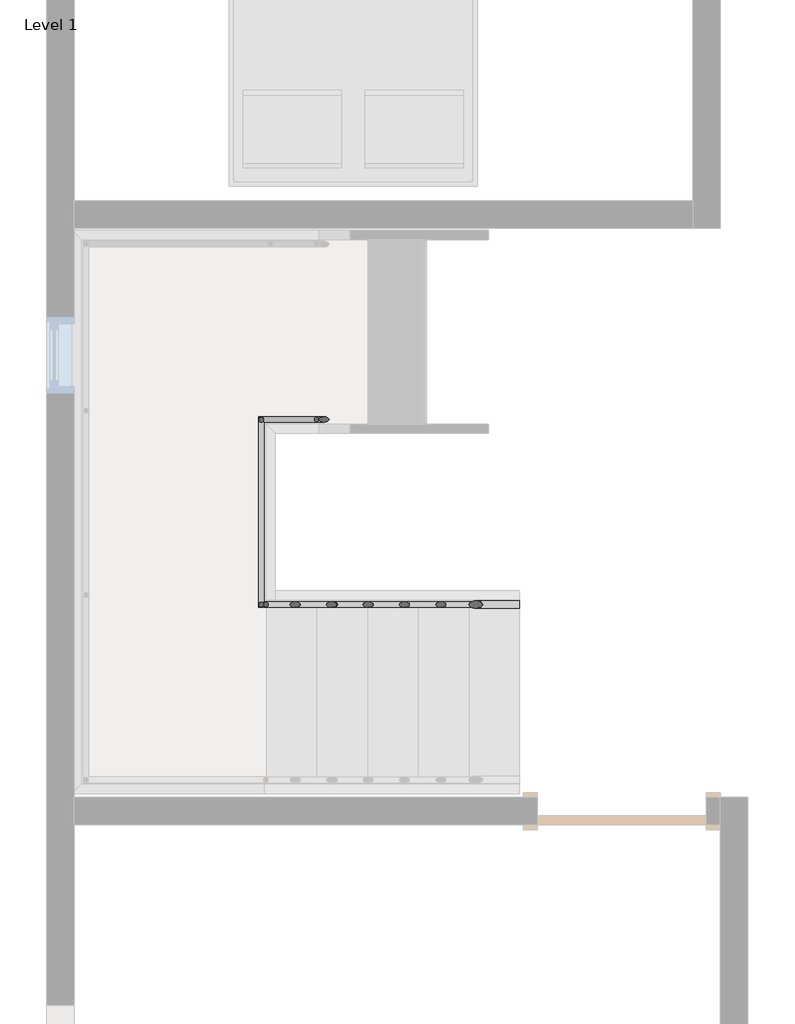
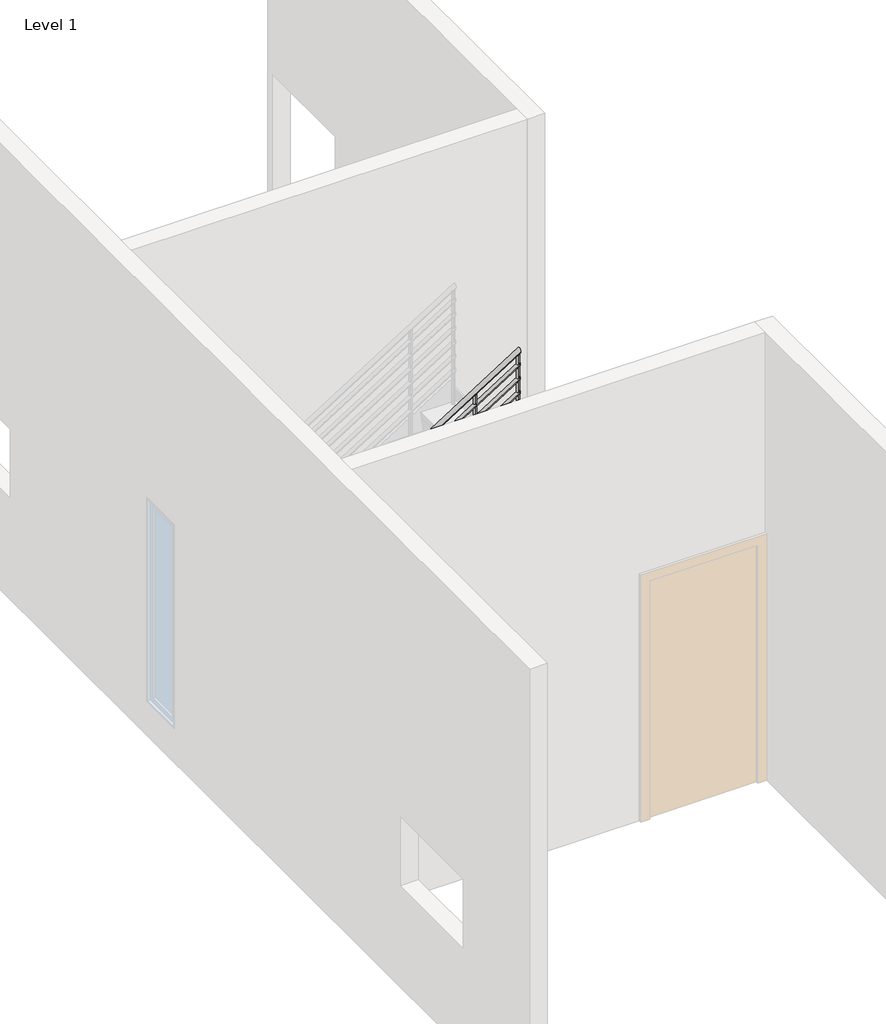
# One storey, part 2 of 4: 1 railing.
"""IFC4 building model written with IfcOpenShell, lengths in millimetres."""

from ifc_helpers import new_model, si_unit, point, frame, frame_2d, origin, place, context, project, spatial, circle_curve, ellipse_curve, trimmed, segment, composite_curve, outline, extrude, element, save
from ifc_brep_helpers import plane_surface, cylinder_surface, advanced_brep

model = new_model("IFC4")

# Units and contexts
model_context = context("Model", 3, world=origin())
ifc_project = project(units=[si_unit("LENGTHUNIT", "METRE", prefix="MILLI")], contexts=[model_context])

# Site, building, storey
site = spatial("IfcSite", under=ifc_project)
building = spatial("IfcBuilding", under=site)
storey = spatial("IfcBuildingStorey", under=building, Name="Level 1", Elevation=0.0)

# Railing
placement = place(None, origin())
element("IfcRailing", 1, ObjectType="900mm Pipe", at=placement, inside=storey, context=model_context, shape_type="SolidModel", body=[
    advanced_brep(
    [(-10589.1151057, 1842.5055917, 1050.2491997), (-10589.1151057, 1802.5055917, 1050.2491997), (-11983.3015939, 1842.5055917, 1931.9481645), (-12017.1084431, 1802.5055917, 1953.3279902)],
    [
        (0, 1, ellipse_curve(frame((-10589.1151057, 1822.5055917, 1050.2491997), z_axis=(1.0, 0.0, 0.0), x_axis=(0.0, 0.0, -1.0)), 23.6638438, 20.0)),
        (1, 0, ellipse_curve(frame((-10589.1151057, 1822.5055917, 1050.2491997), z_axis=(1.0, 0.0, 0.0), x_axis=(0.0, 0.0, -1.0)), 23.6638438, 20.0)),
        (2, 3, ellipse_curve(frame((-12000.2050185, 1822.5055917, 1942.6380773), z_axis=(-0.5976263089853372, 0.7071067811865505, 0.3779454918484384), x_axis=(0.597626308985345, 0.7071067811865446, -0.37794549184843734)), 28.2842712, 20.0)),
        (3, 2, ellipse_curve(frame((-12000.2050185, 1822.5055917, 1942.6380773), z_axis=(-0.5976263089853372, 0.7071067811865505, 0.3779454918484384), x_axis=(0.597626308985345, 0.7071067811865446, -0.37794549184843734)), 28.2842712, 20.0)),
        (0, 2),
        (3, 1),
    ],
    [
        plane_surface(frame((-10589.1151057, 1822.5055917, 1073.9130435), z_axis=(1.0, 0.0, 0.0), x_axis=(0.0, -1.0, 0.0))),
        plane_surface(frame((-11989.5151057, 1822.5055917, 1959.541502), z_axis=(-0.5976263089853373, 0.7071067811865506, 0.3779454918484385), x_axis=(0.8017747781070207, 0.527062745346941, 0.2817127396103761))),
        cylinder_surface(frame((-10599.8050185, 1822.5055917, 1057.0096189), z_axis=(0.8451712313980433, 0.0, -0.5344956404098309), x_axis=(0.0, -1.0, 0.0)), 20.0),
    ],
    [
        (0, [[1, 2]]),
        (1, [[3, 4]]),
        (2, [[-1, 5, -4, 6]]),
        (2, [[-2, -6, -3, -5]]),
    ],
),
    advanced_brep(
    [(-11969.5151057, 1850.0989291, 1923.4782609), (-12009.5151057, 1816.2920799, 1923.4782609), (-11969.5151057, 2805.5398477, 1923.4782609), (-12009.5151057, 2845.5398477, 1923.4782609), (-11683.3216527, 2805.5398477, 1923.4782609), (-11683.3216527, 2845.5398477, 1923.4782609), (-10314.1151057, 2805.5398477, 2789.3796345), (-10314.1151057, 2845.5398477, 2789.3796345)],
    [
        (0, 1, ellipse_curve(frame((-11989.5151057, 1833.1955045, 1923.4782609), z_axis=(0.5976263089853372, -0.7071067811865505, -0.3779454918484384), x_axis=(-0.597626308985345, -0.7071067811865447, 0.37794549184843723)), 28.2842712, 20.0)),
        (1, 0, ellipse_curve(frame((-11989.5151057, 1833.1955045, 1923.4782609), z_axis=(0.5976263089853372, -0.7071067811865505, -0.3779454918484384), x_axis=(-0.597626308985345, -0.7071067811865447, 0.37794549184843723)), 28.2842712, 20.0)),
        (0, 2),
        (2, 3, ellipse_curve(frame((-11989.5151057, 2825.5398477, 1923.4782609), z_axis=(-0.7071067811865511, -0.7071067811865439, 0.0), x_axis=(0.7071067811865437, -0.7071067811865512, 0.0)), 28.2842712, 20.0)),
        (3, 1),
        (3, 2, ellipse_curve(frame((-11989.5151057, 2825.5398477, 1923.4782609), z_axis=(-0.7071067811865511, -0.7071067811865439, 0.0), x_axis=(0.7071067811865437, -0.7071067811865512, 0.0)), 28.2842712, 20.0)),
        (2, 4),
        (4, 5, ellipse_curve(frame((-11683.3216527, 2825.5398477, 1923.4782609), z_axis=(-0.9605132043335073, 0.0, -0.2782344053149753), x_axis=(-0.27823440531497595, 0.0, 0.9605132043335072)), 20.822202, 20.0)),
        (5, 3),
        (5, 4, ellipse_curve(frame((-11683.3216527, 2825.5398477, 1923.4782609), z_axis=(-0.9605132043335073, 0.0, -0.2782344053149753), x_axis=(-0.27823440531497595, 0.0, 0.9605132043335072)), 20.822202, 20.0)),
        (6, 7, ellipse_curve(frame((-10314.1151057, 2825.5398477, 2789.3796345), z_axis=(1.0, 0.0, 0.0), x_axis=(0.0, 0.0, -1.0)), 23.6638438, 20.0)),
        (7, 6, ellipse_curve(frame((-10314.1151057, 2825.5398477, 2789.3796345), z_axis=(1.0, 0.0, 0.0), x_axis=(0.0, 0.0, -1.0)), 23.6638438, 20.0)),
        (4, 6),
        (7, 5),
    ],
    [
        plane_surface(frame((-11989.5151057, 1822.5055917, 1943.4782609), z_axis=(0.5976263089853373, -0.7071067811865506, -0.3779454918484385), x_axis=(0.8017747781070207, 0.527062745346941, 0.2817127396103761))),
        cylinder_surface(frame((-11989.5151057, 1822.5055917, 1923.4782609), z_axis=(0.0, -1.0, 0.0), x_axis=(-1.0, 0.0, 0.0)), 20.0),
        cylinder_surface(frame((-11989.5151057, 2825.5398477, 1923.4782609), z_axis=(-1.0, 0.0, 0.0), x_axis=(0.0, 1.0, 0.0)), 20.0),
        plane_surface(frame((-10314.1151057, 2825.5398477, 2813.0434783), z_axis=(1.0, 0.0, 0.0), x_axis=(0.0, 1.0, 0.0))),
        cylinder_surface(frame((-11678.4251929, 2825.5398477, 1926.5748362), z_axis=(-0.8451712313980441, 0.0, -0.5344956404098296), x_axis=(0.0, 1.0, 0.0)), 20.0),
    ],
    [
        (0, [[1, 2]]),
        (1, [[-1, 3, 4, 5]]),
        (1, [[-2, -5, 6, -3]]),
        (2, [[-4, 7, 8, 9]]),
        (2, [[-6, -9, 10, -7]]),
        (3, [[11, 12]]),
        (4, [[-8, 13, -12, 14]]),
        (4, [[-10, -14, -11, -13]]),
    ],
),
    advanced_brep(
    [(-10589.1151057, 1807.5055917, 931.1651606), (-10589.1151057, 1837.5055917, 931.1651606), (-11968.4601955, 1807.5055917, 1803.4782609), (-11968.4601955, 1837.5055917, 1803.4782609), (-12004.5151057, 1807.5055917, 1803.4782609), (-11974.5151057, 1837.5055917, 1803.4782609), (-12004.5151057, 2840.5398477, 1803.4782609), (-11974.5151057, 2810.5398477, 1803.4782609), (-11684.7700159, 2840.5398477, 1803.4782609), (-11684.7700159, 2810.5398477, 1803.4782609), (-10314.1151057, 2840.5398477, 2670.2955954), (-10314.1151057, 2810.5398477, 2670.2955954)],
    [
        (0, 1, ellipse_curve(frame((-10589.1151057, 1822.5055917, 931.1651606), z_axis=(1.0, 0.0, 0.0), x_axis=(0.0, 0.0, -1.0)), 17.7478828, 15.0)),
        (1, 0, ellipse_curve(frame((-10589.1151057, 1822.5055917, 931.1651606), z_axis=(1.0, 0.0, 0.0), x_axis=(0.0, 0.0, -1.0)), 17.7478828, 15.0)),
        (0, 2),
        (2, 3, ellipse_curve(frame((-11968.4601955, 1822.5055917, 1803.4782609), z_axis=(0.9605132043335071, 0.0, -0.27823440531497595), x_axis=(-0.27823440531497534, 0.0, -0.9605132043335073)), 15.6166515, 15.0)),
        (3, 1),
        (3, 2, ellipse_curve(frame((-11968.4601955, 1822.5055917, 1803.4782609), z_axis=(0.9605132043335071, 0.0, -0.27823440531497595), x_axis=(-0.27823440531497534, 0.0, -0.9605132043335073)), 15.6166515, 15.0)),
        (2, 4),
        (4, 5, ellipse_curve(frame((-11989.5151057, 1822.5055917, 1803.4782609), z_axis=(0.7071067811865439, -0.707106781186551, 0.0), x_axis=(0.7071067811865512, 0.7071067811865438, 0.0)), 21.2132034, 15.0)),
        (5, 3),
        (5, 4, ellipse_curve(frame((-11989.5151057, 1822.5055917, 1803.4782609), z_axis=(0.7071067811865439, -0.707106781186551, 0.0), x_axis=(0.7071067811865512, 0.7071067811865438, 0.0)), 21.2132034, 15.0)),
        (4, 6),
        (6, 7, ellipse_curve(frame((-11989.5151057, 2825.5398477, 1803.4782609), z_axis=(-0.7071067811865511, -0.7071067811865439, 0.0), x_axis=(0.7071067811865439, -0.707106781186551, 0.0)), 21.2132034, 15.0)),
        (7, 5),
        (7, 6, ellipse_curve(frame((-11989.5151057, 2825.5398477, 1803.4782609), z_axis=(-0.7071067811865511, -0.7071067811865439, 0.0), x_axis=(0.7071067811865439, -0.707106781186551, 0.0)), 21.2132034, 15.0)),
        (6, 8),
        (8, 9, ellipse_curve(frame((-11684.7700159, 2825.5398477, 1803.4782609), z_axis=(-0.9605132043335073, 0.0, -0.2782344053149754), x_axis=(-0.2782344053149759, 0.0, 0.9605132043335072)), 15.6166515, 15.0)),
        (9, 7),
        (9, 8, ellipse_curve(frame((-11684.7700159, 2825.5398477, 1803.4782609), z_axis=(-0.9605132043335073, 0.0, -0.2782344053149754), x_axis=(-0.2782344053149759, 0.0, 0.9605132043335072)), 15.6166515, 15.0)),
        (10, 11, ellipse_curve(frame((-10314.1151057, 2825.5398477, 2670.2955954), z_axis=(1.0, 0.0, 0.0), x_axis=(0.0, 0.0, -1.0)), 17.7478828, 15.0)),
        (11, 10, ellipse_curve(frame((-10314.1151057, 2825.5398477, 2670.2955954), z_axis=(1.0, 0.0, 0.0), x_axis=(0.0, 0.0, -1.0)), 17.7478828, 15.0)),
        (8, 10),
        (11, 9),
    ],
    [
        plane_surface(frame((-10589.1151057, 1822.5055917, 948.9130435), z_axis=(1.0, 0.0, 0.0), x_axis=(0.0, -1.0, 0.0))),
        cylinder_surface(frame((-10597.1325403, 1822.5055917, 936.235475), z_axis=(0.8451712313980435, 0.0, -0.5344956404098307), x_axis=(0.0, 1.0, 0.0)), 15.0),
        cylinder_surface(frame((-11964.1151057, 1822.5055917, 1803.4782609), z_axis=(1.0, 0.0, 0.0), x_axis=(0.0, 1.0, 0.0)), 15.0),
        cylinder_surface(frame((-11989.5151057, 1822.5055917, 1803.4782609), z_axis=(0.0, -1.0, 0.0), x_axis=(1.0, 0.0, 0.0)), 15.0),
        cylinder_surface(frame((-11989.5151057, 2825.5398477, 1803.4782609), z_axis=(-1.0, 0.0, 0.0), x_axis=(0.0, -1.0, 0.0)), 15.0),
        plane_surface(frame((-10314.1151057, 2825.5398477, 2688.0434783), z_axis=(1.0, 0.0, 0.0), x_axis=(0.0, 1.0, 0.0))),
        cylinder_surface(frame((-11681.0976711, 2825.5398477, 1805.8006924), z_axis=(-0.845171231398044, 0.0, -0.5344956404098297), x_axis=(0.0, -1.0, 0.0)), 15.0),
    ],
    [
        (0, [[1, 2]]),
        (1, [[-1, 3, 4, 5]]),
        (1, [[-2, -5, 6, -3]]),
        (2, [[-4, 7, 8, 9]]),
        (2, [[-6, -9, 10, -7]]),
        (3, [[-8, 11, 12, 13]]),
        (3, [[-10, -13, 14, -11]]),
        (4, [[-12, 15, 16, 17]]),
        (4, [[-14, -17, 18, -15]]),
        (5, [[19, 20]]),
        (6, [[-16, 21, -20, 22]]),
        (6, [[-18, -22, -19, -21]]),
    ],
),
    advanced_brep(
    [(-10589.1151057, 1807.5055917, 806.1651606), (-10589.1151057, 1837.5055917, 806.1651606), (-11968.4601955, 1807.5055917, 1678.4782609), (-11968.4601955, 1837.5055917, 1678.4782609), (-12004.5151057, 1807.5055917, 1678.4782609), (-11974.5151057, 1837.5055917, 1678.4782609), (-12004.5151057, 2840.5398477, 1678.4782609), (-11974.5151057, 2810.5398477, 1678.4782609), (-11684.7700159, 2840.5398477, 1678.4782609), (-11684.7700159, 2810.5398477, 1678.4782609), (-10314.1151057, 2840.5398477, 2545.2955954), (-10314.1151057, 2810.5398477, 2545.2955954)],
    [
        (0, 1, ellipse_curve(frame((-10589.1151057, 1822.5055917, 806.1651606), z_axis=(1.0, 0.0, 0.0), x_axis=(0.0, 0.0, -1.0)), 17.7478828, 15.0)),
        (1, 0, ellipse_curve(frame((-10589.1151057, 1822.5055917, 806.1651606), z_axis=(1.0, 0.0, 0.0), x_axis=(0.0, 0.0, -1.0)), 17.7478828, 15.0)),
        (0, 2),
        (2, 3, ellipse_curve(frame((-11968.4601955, 1822.5055917, 1678.4782609), z_axis=(0.9605132043335073, 0.0, -0.2782344053149759), x_axis=(-0.2782344053149766, 0.0, -0.960513204333507)), 15.6166515, 15.0)),
        (3, 1),
        (3, 2, ellipse_curve(frame((-11968.4601955, 1822.5055917, 1678.4782609), z_axis=(0.9605132043335073, 0.0, -0.2782344053149759), x_axis=(-0.2782344053149766, 0.0, -0.960513204333507)), 15.6166515, 15.0)),
        (2, 4),
        (4, 5, ellipse_curve(frame((-11989.5151057, 1822.5055917, 1678.4782609), z_axis=(0.7071067811865439, -0.707106781186551, 0.0), x_axis=(0.7071067811865512, 0.7071067811865438, 0.0)), 21.2132034, 15.0)),
        (5, 3),
        (5, 4, ellipse_curve(frame((-11989.5151057, 1822.5055917, 1678.4782609), z_axis=(0.7071067811865439, -0.707106781186551, 0.0), x_axis=(0.7071067811865512, 0.7071067811865438, 0.0)), 21.2132034, 15.0)),
        (4, 6),
        (6, 7, ellipse_curve(frame((-11989.5151057, 2825.5398477, 1678.4782609), z_axis=(-0.7071067811865511, -0.7071067811865439, 0.0), x_axis=(0.7071067811865439, -0.707106781186551, 0.0)), 21.2132034, 15.0)),
        (7, 5),
        (7, 6, ellipse_curve(frame((-11989.5151057, 2825.5398477, 1678.4782609), z_axis=(-0.7071067811865511, -0.7071067811865439, 0.0), x_axis=(0.7071067811865439, -0.707106781186551, 0.0)), 21.2132034, 15.0)),
        (6, 8),
        (8, 9, ellipse_curve(frame((-11684.7700159, 2825.5398477, 1678.4782609), z_axis=(-0.9605132043335073, 0.0, -0.2782344053149753), x_axis=(-0.278234405314976, 0.0, 0.9605132043335073)), 15.6166515, 15.0)),
        (9, 7),
        (9, 8, ellipse_curve(frame((-11684.7700159, 2825.5398477, 1678.4782609), z_axis=(-0.9605132043335073, 0.0, -0.2782344053149753), x_axis=(-0.278234405314976, 0.0, 0.9605132043335073)), 15.6166515, 15.0)),
        (10, 11, ellipse_curve(frame((-10314.1151057, 2825.5398477, 2545.2955954), z_axis=(1.0, 0.0, 0.0), x_axis=(0.0, 0.0, -1.0)), 17.7478828, 15.0)),
        (11, 10, ellipse_curve(frame((-10314.1151057, 2825.5398477, 2545.2955954), z_axis=(1.0, 0.0, 0.0), x_axis=(0.0, 0.0, -1.0)), 17.7478828, 15.0)),
        (8, 10),
        (11, 9),
    ],
    [
        plane_surface(frame((-10589.1151057, 1822.5055917, 823.9130435), z_axis=(1.0, 0.0, 0.0), x_axis=(0.0, -1.0, 0.0))),
        cylinder_surface(frame((-10597.1325403, 1822.5055917, 811.235475), z_axis=(0.8451712313980436, 0.0, -0.5344956404098306), x_axis=(0.0, 1.0, 0.0)), 15.0),
        cylinder_surface(frame((-11964.1151057, 1822.5055917, 1678.4782609), z_axis=(1.0, 0.0, 0.0), x_axis=(0.0, 1.0, 0.0)), 15.0),
        cylinder_surface(frame((-11989.5151057, 1822.5055917, 1678.4782609), z_axis=(0.0, -1.0, 0.0), x_axis=(1.0, 0.0, 0.0)), 15.0),
        cylinder_surface(frame((-11989.5151057, 2825.5398477, 1678.4782609), z_axis=(-1.0, 0.0, 0.0), x_axis=(0.0, -1.0, 0.0)), 15.0),
        plane_surface(frame((-10314.1151057, 2825.5398477, 2563.0434783), z_axis=(1.0, 0.0, 0.0), x_axis=(0.0, 1.0, 0.0))),
        cylinder_surface(frame((-11681.0976711, 2825.5398477, 1680.8006924), z_axis=(-0.8451712313980441, 0.0, -0.5344956404098296), x_axis=(0.0, -1.0, 0.0)), 15.0),
    ],
    [
        (0, [[1, 2]]),
        (1, [[-1, 3, 4, 5]]),
        (1, [[-2, -5, 6, -3]]),
        (2, [[-4, 7, 8, 9]]),
        (2, [[-6, -9, 10, -7]]),
        (3, [[-8, 11, 12, 13]]),
        (3, [[-10, -13, 14, -11]]),
        (4, [[-12, 15, 16, 17]]),
        (4, [[-14, -17, 18, -15]]),
        (5, [[19, 20]]),
        (6, [[-16, 21, -20, 22]]),
        (6, [[-18, -22, -19, -21]]),
    ],
),
    advanced_brep(
    [(-10589.1151057, 1807.5055917, 681.1651606), (-10589.1151057, 1837.5055917, 681.1651606), (-11968.4601955, 1807.5055917, 1553.4782609), (-11968.4601955, 1837.5055917, 1553.4782609), (-12004.5151057, 1807.5055917, 1553.4782609), (-11974.5151057, 1837.5055917, 1553.4782609), (-12004.5151057, 2840.5398477, 1553.4782609), (-11974.5151057, 2810.5398477, 1553.4782609), (-11684.7700159, 2840.5398477, 1553.4782609), (-11684.7700159, 2810.5398477, 1553.4782609), (-10314.1151057, 2840.5398477, 2420.2955954), (-10314.1151057, 2810.5398477, 2420.2955954)],
    [
        (0, 1, ellipse_curve(frame((-10589.1151057, 1822.5055917, 681.1651606), z_axis=(1.0, 0.0, 0.0), x_axis=(0.0, 0.0, -1.0)), 17.7478828, 15.0)),
        (1, 0, ellipse_curve(frame((-10589.1151057, 1822.5055917, 681.1651606), z_axis=(1.0, 0.0, 0.0), x_axis=(0.0, 0.0, -1.0)), 17.7478828, 15.0)),
        (0, 2),
        (2, 3, ellipse_curve(frame((-11968.4601955, 1822.5055917, 1553.4782609), z_axis=(0.9605132043335071, 0.0, -0.27823440531497595), x_axis=(-0.27823440531497534, 0.0, -0.9605132043335073)), 15.6166515, 15.0)),
        (3, 1),
        (3, 2, ellipse_curve(frame((-11968.4601955, 1822.5055917, 1553.4782609), z_axis=(0.9605132043335071, 0.0, -0.27823440531497595), x_axis=(-0.27823440531497534, 0.0, -0.9605132043335073)), 15.6166515, 15.0)),
        (2, 4),
        (4, 5, ellipse_curve(frame((-11989.5151057, 1822.5055917, 1553.4782609), z_axis=(0.7071067811865439, -0.707106781186551, 0.0), x_axis=(0.7071067811865512, 0.7071067811865438, 0.0)), 21.2132034, 15.0)),
        (5, 3),
        (5, 4, ellipse_curve(frame((-11989.5151057, 1822.5055917, 1553.4782609), z_axis=(0.7071067811865439, -0.707106781186551, 0.0), x_axis=(0.7071067811865512, 0.7071067811865438, 0.0)), 21.2132034, 15.0)),
        (4, 6),
        (6, 7, ellipse_curve(frame((-11989.5151057, 2825.5398477, 1553.4782609), z_axis=(-0.7071067811865511, -0.7071067811865439, 0.0), x_axis=(0.7071067811865439, -0.707106781186551, 0.0)), 21.2132034, 15.0)),
        (7, 5),
        (7, 6, ellipse_curve(frame((-11989.5151057, 2825.5398477, 1553.4782609), z_axis=(-0.7071067811865511, -0.7071067811865439, 0.0), x_axis=(0.7071067811865439, -0.707106781186551, 0.0)), 21.2132034, 15.0)),
        (6, 8),
        (8, 9, ellipse_curve(frame((-11684.7700159, 2825.5398477, 1553.4782609), z_axis=(-0.9605132043335073, 0.0, -0.2782344053149754), x_axis=(-0.2782344053149759, 0.0, 0.9605132043335072)), 15.6166515, 15.0)),
        (9, 7),
        (9, 8, ellipse_curve(frame((-11684.7700159, 2825.5398477, 1553.4782609), z_axis=(-0.9605132043335073, 0.0, -0.2782344053149754), x_axis=(-0.2782344053149759, 0.0, 0.9605132043335072)), 15.6166515, 15.0)),
        (10, 11, ellipse_curve(frame((-10314.1151057, 2825.5398477, 2420.2955954), z_axis=(1.0, 0.0, 0.0), x_axis=(0.0, 0.0, -1.0)), 17.7478828, 15.0)),
        (11, 10, ellipse_curve(frame((-10314.1151057, 2825.5398477, 2420.2955954), z_axis=(1.0, 0.0, 0.0), x_axis=(0.0, 0.0, -1.0)), 17.7478828, 15.0)),
        (8, 10),
        (11, 9),
    ],
    [
        plane_surface(frame((-10589.1151057, 1822.5055917, 698.9130435), z_axis=(1.0, 0.0, 0.0), x_axis=(0.0, -1.0, 0.0))),
        cylinder_surface(frame((-10597.1325403, 1822.5055917, 686.235475), z_axis=(0.8451712313980435, 0.0, -0.5344956404098307), x_axis=(0.0, 1.0, 0.0)), 15.0),
        cylinder_surface(frame((-11964.1151057, 1822.5055917, 1553.4782609), z_axis=(1.0, 0.0, 0.0), x_axis=(0.0, 1.0, 0.0)), 15.0),
        cylinder_surface(frame((-11989.5151057, 1822.5055917, 1553.4782609), z_axis=(0.0, -1.0, 0.0), x_axis=(1.0, 0.0, 0.0)), 15.0),
        cylinder_surface(frame((-11989.5151057, 2825.5398477, 1553.4782609), z_axis=(-1.0, 0.0, 0.0), x_axis=(0.0, -1.0, 0.0)), 15.0),
        plane_surface(frame((-10314.1151057, 2825.5398477, 2438.0434783), z_axis=(1.0, 0.0, 0.0), x_axis=(0.0, 1.0, 0.0))),
        cylinder_surface(frame((-11681.0976711, 2825.5398477, 1555.8006924), z_axis=(-0.845171231398044, 0.0, -0.5344956404098297), x_axis=(0.0, -1.0, 0.0)), 15.0),
    ],
    [
        (0, [[1, 2]]),
        (1, [[-1, 3, 4, 5]]),
        (1, [[-2, -5, 6, -3]]),
        (2, [[-4, 7, 8, 9]]),
        (2, [[-6, -9, 10, -7]]),
        (3, [[-8, 11, 12, 13]]),
        (3, [[-10, -13, 14, -11]]),
        (4, [[-12, 15, 16, 17]]),
        (4, [[-14, -17, 18, -15]]),
        (5, [[19, 20]]),
        (6, [[-16, 21, -20, 22]]),
        (6, [[-18, -22, -19, -21]]),
    ],
),
    advanced_brep(
    [(-10589.1151057, 1807.5055917, 556.1651606), (-10589.1151057, 1837.5055917, 556.1651606), (-11968.4601955, 1807.5055917, 1428.4782609), (-11968.4601955, 1837.5055917, 1428.4782609), (-12004.5151057, 1807.5055917, 1428.4782609), (-11974.5151057, 1837.5055917, 1428.4782609), (-12004.5151057, 2840.5398477, 1428.4782609), (-11974.5151057, 2810.5398477, 1428.4782609), (-11684.7700159, 2840.5398477, 1428.4782609), (-11684.7700159, 2810.5398477, 1428.4782609), (-10314.1151057, 2840.5398477, 2295.2955954), (-10314.1151057, 2810.5398477, 2295.2955954)],
    [
        (0, 1, ellipse_curve(frame((-10589.1151057, 1822.5055917, 556.1651606), z_axis=(1.0, 0.0, 0.0), x_axis=(0.0, 0.0, -1.0)), 17.7478828, 15.0)),
        (1, 0, ellipse_curve(frame((-10589.1151057, 1822.5055917, 556.1651606), z_axis=(1.0, 0.0, 0.0), x_axis=(0.0, 0.0, -1.0)), 17.7478828, 15.0)),
        (0, 2),
        (2, 3, ellipse_curve(frame((-11968.4601955, 1822.5055917, 1428.4782609), z_axis=(0.9605132043335073, 0.0, -0.2782344053149759), x_axis=(-0.2782344053149766, 0.0, -0.960513204333507)), 15.6166515, 15.0)),
        (3, 1),
        (3, 2, ellipse_curve(frame((-11968.4601955, 1822.5055917, 1428.4782609), z_axis=(0.9605132043335073, 0.0, -0.2782344053149759), x_axis=(-0.2782344053149766, 0.0, -0.960513204333507)), 15.6166515, 15.0)),
        (2, 4),
        (4, 5, ellipse_curve(frame((-11989.5151057, 1822.5055917, 1428.4782609), z_axis=(0.7071067811865439, -0.707106781186551, 0.0), x_axis=(0.7071067811865512, 0.7071067811865438, 0.0)), 21.2132034, 15.0)),
        (5, 3),
        (5, 4, ellipse_curve(frame((-11989.5151057, 1822.5055917, 1428.4782609), z_axis=(0.7071067811865439, -0.707106781186551, 0.0), x_axis=(0.7071067811865512, 0.7071067811865438, 0.0)), 21.2132034, 15.0)),
        (4, 6),
        (6, 7, ellipse_curve(frame((-11989.5151057, 2825.5398477, 1428.4782609), z_axis=(-0.7071067811865511, -0.7071067811865439, 0.0), x_axis=(0.7071067811865439, -0.707106781186551, 0.0)), 21.2132034, 15.0)),
        (7, 5),
        (7, 6, ellipse_curve(frame((-11989.5151057, 2825.5398477, 1428.4782609), z_axis=(-0.7071067811865511, -0.7071067811865439, 0.0), x_axis=(0.7071067811865439, -0.707106781186551, 0.0)), 21.2132034, 15.0)),
        (6, 8),
        (8, 9, ellipse_curve(frame((-11684.7700159, 2825.5398477, 1428.4782609), z_axis=(-0.9605132043335073, 0.0, -0.27823440531497534), x_axis=(-0.27823440531497595, 0.0, 0.9605132043335072)), 15.6166515, 15.0)),
        (9, 7),
        (9, 8, ellipse_curve(frame((-11684.7700159, 2825.5398477, 1428.4782609), z_axis=(-0.9605132043335073, 0.0, -0.27823440531497534), x_axis=(-0.27823440531497595, 0.0, 0.9605132043335072)), 15.6166515, 15.0)),
        (10, 11, ellipse_curve(frame((-10314.1151057, 2825.5398477, 2295.2955954), z_axis=(1.0, 0.0, 0.0), x_axis=(0.0, 0.0, -1.0)), 17.7478828, 15.0)),
        (11, 10, ellipse_curve(frame((-10314.1151057, 2825.5398477, 2295.2955954), z_axis=(1.0, 0.0, 0.0), x_axis=(0.0, 0.0, -1.0)), 17.7478828, 15.0)),
        (8, 10),
        (11, 9),
    ],
    [
        plane_surface(frame((-10589.1151057, 1822.5055917, 573.9130435), z_axis=(1.0, 0.0, 0.0), x_axis=(0.0, -1.0, 0.0))),
        cylinder_surface(frame((-10597.1325403, 1822.5055917, 561.235475), z_axis=(0.8451712313980436, 0.0, -0.5344956404098306), x_axis=(0.0, 1.0, 0.0)), 15.0),
        cylinder_surface(frame((-11964.1151057, 1822.5055917, 1428.4782609), z_axis=(1.0, 0.0, 0.0), x_axis=(0.0, 1.0, 0.0)), 15.0),
        cylinder_surface(frame((-11989.5151057, 1822.5055917, 1428.4782609), z_axis=(0.0, -1.0, 0.0), x_axis=(1.0, 0.0, 0.0)), 15.0),
        cylinder_surface(frame((-11989.5151057, 2825.5398477, 1428.4782609), z_axis=(-1.0, 0.0, 0.0), x_axis=(0.0, -1.0, 0.0)), 15.0),
        plane_surface(frame((-10314.1151057, 2825.5398477, 2313.0434783), z_axis=(1.0, 0.0, 0.0), x_axis=(0.0, 1.0, 0.0))),
        cylinder_surface(frame((-11681.0976711, 2825.5398477, 1430.8006924), z_axis=(-0.845171231398044, 0.0, -0.5344956404098297), x_axis=(0.0, -1.0, 0.0)), 15.0),
    ],
    [
        (0, [[1, 2]]),
        (1, [[-1, 3, 4, 5]]),
        (1, [[-2, -5, 6, -3]]),
        (2, [[-4, 7, 8, 9]]),
        (2, [[-6, -9, 10, -7]]),
        (3, [[-8, 11, 12, 13]]),
        (3, [[-10, -13, 14, -11]]),
        (4, [[-12, 15, 16, 17]]),
        (4, [[-14, -17, 18, -15]]),
        (5, [[19, 20]]),
        (6, [[-16, 21, -20, 22]]),
        (6, [[-18, -22, -19, -21]]),
    ],
),
    advanced_brep(
    [(-10589.1151057, 1807.5055917, 431.1651606), (-10589.1151057, 1837.5055917, 431.1651606), (-11968.4601955, 1807.5055917, 1303.4782609), (-11968.4601955, 1837.5055917, 1303.4782609), (-12004.5151057, 1807.5055917, 1303.4782609), (-11974.5151057, 1837.5055917, 1303.4782609), (-12004.5151057, 2840.5398477, 1303.4782609), (-11974.5151057, 2810.5398477, 1303.4782609), (-11684.7700159, 2840.5398477, 1303.4782609), (-11684.7700159, 2810.5398477, 1303.4782609), (-10314.1151057, 2840.5398477, 2170.2955954), (-10314.1151057, 2810.5398477, 2170.2955954)],
    [
        (0, 1, ellipse_curve(frame((-10589.1151057, 1822.5055917, 431.1651606), z_axis=(1.0, 0.0, 0.0), x_axis=(0.0, 0.0, -1.0)), 17.7478828, 15.0)),
        (1, 0, ellipse_curve(frame((-10589.1151057, 1822.5055917, 431.1651606), z_axis=(1.0, 0.0, 0.0), x_axis=(0.0, 0.0, -1.0)), 17.7478828, 15.0)),
        (0, 2),
        (2, 3, ellipse_curve(frame((-11968.4601955, 1822.5055917, 1303.4782609), z_axis=(0.9605132043335071, 0.0, -0.27823440531497595), x_axis=(-0.27823440531497534, 0.0, -0.9605132043335073)), 15.6166515, 15.0)),
        (3, 1),
        (3, 2, ellipse_curve(frame((-11968.4601955, 1822.5055917, 1303.4782609), z_axis=(0.9605132043335071, 0.0, -0.27823440531497595), x_axis=(-0.27823440531497534, 0.0, -0.9605132043335073)), 15.6166515, 15.0)),
        (2, 4),
        (4, 5, ellipse_curve(frame((-11989.5151057, 1822.5055917, 1303.4782609), z_axis=(0.7071067811865439, -0.707106781186551, 0.0), x_axis=(0.7071067811865512, 0.7071067811865438, 0.0)), 21.2132034, 15.0)),
        (5, 3),
        (5, 4, ellipse_curve(frame((-11989.5151057, 1822.5055917, 1303.4782609), z_axis=(0.7071067811865439, -0.707106781186551, 0.0), x_axis=(0.7071067811865512, 0.7071067811865438, 0.0)), 21.2132034, 15.0)),
        (4, 6),
        (6, 7, ellipse_curve(frame((-11989.5151057, 2825.5398477, 1303.4782609), z_axis=(-0.7071067811865511, -0.7071067811865439, 0.0), x_axis=(0.7071067811865439, -0.707106781186551, 0.0)), 21.2132034, 15.0)),
        (7, 5),
        (7, 6, ellipse_curve(frame((-11989.5151057, 2825.5398477, 1303.4782609), z_axis=(-0.7071067811865511, -0.7071067811865439, 0.0), x_axis=(0.7071067811865439, -0.707106781186551, 0.0)), 21.2132034, 15.0)),
        (6, 8),
        (8, 9, ellipse_curve(frame((-11684.7700159, 2825.5398477, 1303.4782609), z_axis=(-0.9605132043335073, 0.0, -0.2782344053149754), x_axis=(-0.2782344053149759, 0.0, 0.9605132043335072)), 15.6166515, 15.0)),
        (9, 7),
        (9, 8, ellipse_curve(frame((-11684.7700159, 2825.5398477, 1303.4782609), z_axis=(-0.9605132043335073, 0.0, -0.2782344053149754), x_axis=(-0.2782344053149759, 0.0, 0.9605132043335072)), 15.6166515, 15.0)),
        (10, 11, ellipse_curve(frame((-10314.1151057, 2825.5398477, 2170.2955954), z_axis=(1.0, 0.0, 0.0), x_axis=(0.0, 0.0, -1.0)), 17.7478828, 15.0)),
        (11, 10, ellipse_curve(frame((-10314.1151057, 2825.5398477, 2170.2955954), z_axis=(1.0, 0.0, 0.0), x_axis=(0.0, 0.0, -1.0)), 17.7478828, 15.0)),
        (8, 10),
        (11, 9),
    ],
    [
        plane_surface(frame((-10589.1151057, 1822.5055917, 448.9130435), z_axis=(1.0, 0.0, 0.0), x_axis=(0.0, -1.0, 0.0))),
        cylinder_surface(frame((-10597.1325403, 1822.5055917, 436.235475), z_axis=(0.8451712313980435, 0.0, -0.5344956404098307), x_axis=(0.0, 1.0, 0.0)), 15.0),
        cylinder_surface(frame((-11964.1151057, 1822.5055917, 1303.4782609), z_axis=(1.0, 0.0, 0.0), x_axis=(0.0, 1.0, 0.0)), 15.0),
        cylinder_surface(frame((-11989.5151057, 1822.5055917, 1303.4782609), z_axis=(0.0, -1.0, 0.0), x_axis=(1.0, 0.0, 0.0)), 15.0),
        cylinder_surface(frame((-11989.5151057, 2825.5398477, 1303.4782609), z_axis=(-1.0, 0.0, 0.0), x_axis=(0.0, -1.0, 0.0)), 15.0),
        plane_surface(frame((-10314.1151057, 2825.5398477, 2188.0434783), z_axis=(1.0, 0.0, 0.0), x_axis=(0.0, 1.0, 0.0))),
        cylinder_surface(frame((-11681.0976711, 2825.5398477, 1305.8006924), z_axis=(-0.845171231398044, 0.0, -0.5344956404098297), x_axis=(0.0, -1.0, 0.0)), 15.0),
    ],
    [
        (0, [[1, 2]]),
        (1, [[-1, 3, 4, 5]]),
        (1, [[-2, -5, 6, -3]]),
        (2, [[-4, 7, 8, 9]]),
        (2, [[-6, -9, 10, -7]]),
        (3, [[-8, 11, 12, 13]]),
        (3, [[-10, -13, 14, -11]]),
        (4, [[-12, 15, 16, 17]]),
        (4, [[-14, -17, 18, -15]]),
        (5, [[19, 20]]),
        (6, [[-16, 21, -20, 22]]),
        (6, [[-18, -22, -19, -21]]),
    ],
),
    advanced_brep(
    [(-10589.1151057, 1807.5055917, 306.1651606), (-10589.1151057, 1837.5055917, 306.1651606), (-11968.4601955, 1807.5055917, 1178.4782609), (-11968.4601955, 1837.5055917, 1178.4782609), (-12004.5151057, 1807.5055917, 1178.4782609), (-11974.5151057, 1837.5055917, 1178.4782609), (-12004.5151057, 2840.5398477, 1178.4782609), (-11974.5151057, 2810.5398477, 1178.4782609), (-11684.7700159, 2840.5398477, 1178.4782609), (-11684.7700159, 2810.5398477, 1178.4782609), (-10314.1151057, 2840.5398477, 2045.2955954), (-10314.1151057, 2810.5398477, 2045.2955954)],
    [
        (0, 1, ellipse_curve(frame((-10589.1151057, 1822.5055917, 306.1651606), z_axis=(1.0, 0.0, 0.0), x_axis=(0.0, 0.0, -1.0)), 17.7478828, 15.0)),
        (1, 0, ellipse_curve(frame((-10589.1151057, 1822.5055917, 306.1651606), z_axis=(1.0, 0.0, 0.0), x_axis=(0.0, 0.0, -1.0)), 17.7478828, 15.0)),
        (0, 2),
        (2, 3, ellipse_curve(frame((-11968.4601955, 1822.5055917, 1178.4782609), z_axis=(0.9605132043335073, 0.0, -0.2782344053149759), x_axis=(-0.2782344053149766, 0.0, -0.960513204333507)), 15.6166515, 15.0)),
        (3, 1),
        (3, 2, ellipse_curve(frame((-11968.4601955, 1822.5055917, 1178.4782609), z_axis=(0.9605132043335073, 0.0, -0.2782344053149759), x_axis=(-0.2782344053149766, 0.0, -0.960513204333507)), 15.6166515, 15.0)),
        (2, 4),
        (4, 5, ellipse_curve(frame((-11989.5151057, 1822.5055917, 1178.4782609), z_axis=(0.7071067811865439, -0.707106781186551, 0.0), x_axis=(0.7071067811865512, 0.7071067811865438, 0.0)), 21.2132034, 15.0)),
        (5, 3),
        (5, 4, ellipse_curve(frame((-11989.5151057, 1822.5055917, 1178.4782609), z_axis=(0.7071067811865439, -0.707106781186551, 0.0), x_axis=(0.7071067811865512, 0.7071067811865438, 0.0)), 21.2132034, 15.0)),
        (4, 6),
        (6, 7, ellipse_curve(frame((-11989.5151057, 2825.5398477, 1178.4782609), z_axis=(-0.7071067811865511, -0.7071067811865439, 0.0), x_axis=(0.7071067811865439, -0.707106781186551, 0.0)), 21.2132034, 15.0)),
        (7, 5),
        (7, 6, ellipse_curve(frame((-11989.5151057, 2825.5398477, 1178.4782609), z_axis=(-0.7071067811865511, -0.7071067811865439, 0.0), x_axis=(0.7071067811865439, -0.707106781186551, 0.0)), 21.2132034, 15.0)),
        (6, 8),
        (8, 9, ellipse_curve(frame((-11684.7700159, 2825.5398477, 1178.4782609), z_axis=(-0.9605132043335073, 0.0, -0.27823440531497534), x_axis=(-0.27823440531497595, 0.0, 0.9605132043335072)), 15.6166515, 15.0)),
        (9, 7),
        (9, 8, ellipse_curve(frame((-11684.7700159, 2825.5398477, 1178.4782609), z_axis=(-0.9605132043335073, 0.0, -0.27823440531497534), x_axis=(-0.27823440531497595, 0.0, 0.9605132043335072)), 15.6166515, 15.0)),
        (10, 11, ellipse_curve(frame((-10314.1151057, 2825.5398477, 2045.2955954), z_axis=(1.0, 0.0, 0.0), x_axis=(0.0, 0.0, -1.0)), 17.7478828, 15.0)),
        (11, 10, ellipse_curve(frame((-10314.1151057, 2825.5398477, 2045.2955954), z_axis=(1.0, 0.0, 0.0), x_axis=(0.0, 0.0, -1.0)), 17.7478828, 15.0)),
        (8, 10),
        (11, 9),
    ],
    [
        plane_surface(frame((-10589.1151057, 1822.5055917, 323.9130435), z_axis=(1.0, 0.0, 0.0), x_axis=(0.0, -1.0, 0.0))),
        cylinder_surface(frame((-10597.1325403, 1822.5055917, 311.235475), z_axis=(0.8451712313980436, 0.0, -0.5344956404098306), x_axis=(0.0, 1.0, 0.0)), 15.0),
        cylinder_surface(frame((-11964.1151057, 1822.5055917, 1178.4782609), z_axis=(1.0, 0.0, 0.0), x_axis=(0.0, 1.0, 0.0)), 15.0),
        cylinder_surface(frame((-11989.5151057, 1822.5055917, 1178.4782609), z_axis=(0.0, -1.0, 0.0), x_axis=(1.0, 0.0, 0.0)), 15.0),
        cylinder_surface(frame((-11989.5151057, 2825.5398477, 1178.4782609), z_axis=(-1.0, 0.0, 0.0), x_axis=(0.0, -1.0, 0.0)), 15.0),
        plane_surface(frame((-10314.1151057, 2825.5398477, 2063.0434783), z_axis=(1.0, 0.0, 0.0), x_axis=(0.0, 1.0, 0.0))),
        cylinder_surface(frame((-11681.0976711, 2825.5398477, 1180.8006924), z_axis=(-0.845171231398044, 0.0, -0.5344956404098297), x_axis=(0.0, -1.0, 0.0)), 15.0),
    ],
    [
        (0, [[1, 2]]),
        (1, [[-1, 3, 4, 5]]),
        (1, [[-2, -5, 6, -3]]),
        (2, [[-4, 7, 8, 9]]),
        (2, [[-6, -9, 10, -7]]),
        (3, [[-8, 11, 12, 13]]),
        (3, [[-10, -13, 14, -11]]),
        (4, [[-12, 15, 16, 17]]),
        (4, [[-14, -17, 18, -15]]),
        (5, [[19, 20]]),
        (6, [[-16, 21, -20, 22]]),
        (6, [[-18, -22, -19, -21]]),
    ],
),
    advanced_brep(
    [(-10689.1151057, 2813.0398477, 2528.5616405), (-10689.1151057, 2813.0398477, 1565.2173913), (-10689.1151057, 2838.0398477, 1565.2173913), (-10689.1151057, 2838.0398477, 2528.5616405)],
    [
        (0, 1),
        (1, 2, circle_curve(frame((-10689.1151057, 2825.5398477, 1565.2173913), z_axis=(0.0, 0.0, 1.0), x_axis=(0.0, 1.0, 0.0)), 12.5)),
        (2, 3),
        (3, 0, ellipse_curve(frame((-10689.1151057, 2825.5398477, 2528.5616405), z_axis=(0.5344956404098302, 0.0, -0.8451712313980437), x_axis=(0.8451712313980437, 0.0, 0.53449564040983)), 14.7899024, 12.5)),
        (0, 3, ellipse_curve(frame((-10689.1151057, 2825.5398477, 2528.5616405), z_axis=(0.5344956404098302, 0.0, -0.8451712313980437), x_axis=(0.8451712313980437, 0.0, 0.53449564040983)), 14.7899024, 12.5)),
        (2, 1, circle_curve(frame((-10689.1151057, 2825.5398477, 1565.2173913), z_axis=(0.0, 0.0, 1.0), x_axis=(0.0, 1.0, 0.0)), 12.5)),
    ],
    [
        cylinder_surface(frame((-10689.1151057, 2825.5398477, 1465.2173913), z_axis=(0.0, 0.0, 1.0), x_axis=(0.0, 1.0, 0.0)), 12.5),
        plane_surface(frame((-10664.1151057, 2850.5398477, 2544.3719172), z_axis=(-0.5344956404098302, 0.0, 0.8451712313980437), x_axis=(0.0, -1.0, 0.0))),
        plane_surface(frame((-10714.1151057, 2850.5398477, 1565.2173913), z_axis=(0.0, 0.0, -1.0), x_axis=(0.0, -1.0, 0.0))),
    ],
    [
        (0, [[1, 2, 3, 4]]),
        (0, [[-1, 5, -3, 6]]),
        (1, [[-4, -5]]),
        (2, [[-2, -6]]),
    ],
),
    extrude(outline(composite_curve([segment(trimmed(circle_curve(frame_2d((-11989.5151057, 2822.5055917)), 12.5), [point((-12002.0151057, 2822.5055917))], [point((-11977.0151057, 2822.5055917))], False, "CARTESIAN"), True, "CONTINUOUS"), segment(trimmed(circle_curve(frame_2d((-11989.5151057, 2822.5055917)), 12.5), [point((-11977.0151057, 2822.5055917))], [point((-12002.0151057, 2822.5055917))], False, "CARTESIAN"), True, "CONTINUOUS")], self_intersect=False)), frame((0.0, 0.0, 1043.4782609), z_axis=(0.0, 0.0, 1.0), x_axis=(1.0, 0.0, 0.0)), (0.0, 0.0, 1.0), 860.0),
    advanced_brep(
    [(-11589.1151057, 1835.0055917, 1658.9964231), (-11589.1151057, 1835.0055917, 695.6521739), (-11589.1151057, 1810.0055917, 695.6521739), (-11589.1151057, 1810.0055917, 1658.9964231)],
    [
        (0, 1),
        (1, 2, circle_curve(frame((-11589.1151057, 1822.5055917, 695.6521739), z_axis=(0.0, 0.0, 1.0), x_axis=(0.0, -1.0, 0.0)), 12.5)),
        (2, 3),
        (3, 0, ellipse_curve(frame((-11589.1151057, 1822.5055917, 1658.9964231), z_axis=(-0.5344956404098302, 0.0, -0.8451712313980437), x_axis=(-0.8451712313980437, 0.0, 0.53449564040983)), 14.7899024, 12.5)),
        (0, 3, ellipse_curve(frame((-11589.1151057, 1822.5055917, 1658.9964231), z_axis=(-0.5344956404098302, 0.0, -0.8451712313980437), x_axis=(-0.8451712313980437, 0.0, 0.53449564040983)), 14.7899024, 12.5)),
        (2, 1, circle_curve(frame((-11589.1151057, 1822.5055917, 695.6521739), z_axis=(0.0, 0.0, 1.0), x_axis=(0.0, -1.0, 0.0)), 12.5)),
    ],
    [
        cylinder_surface(frame((-11589.1151057, 1822.5055917, 595.6521739), z_axis=(0.0, 0.0, 1.0), x_axis=(0.0, -1.0, 0.0)), 12.5),
        plane_surface(frame((-11614.1151057, 1797.5055917, 1674.8066998), z_axis=(0.5344956404098302, 0.0, 0.8451712313980437), x_axis=(0.0, 1.0, 0.0))),
        plane_surface(frame((-11564.1151057, 1797.5055917, 695.6521739), z_axis=(0.0, 0.0, -1.0), x_axis=(0.0, 1.0, 0.0))),
    ],
    [
        (0, [[1, 2, 3, 4]]),
        (0, [[-1, 5, -3, 6]]),
        (1, [[-4, -5]]),
        (2, [[-2, -6]]),
    ],
),
    extrude(outline(composite_curve([segment(trimmed(circle_curve(frame_2d((-11689.1151057, 2825.5398477)), 12.5), [point((-11689.1151057, 2838.0398477))], [point((-11689.1151057, 2813.0398477))], False, "CARTESIAN"), True, "CONTINUOUS"), segment(trimmed(circle_curve(frame_2d((-11689.1151057, 2825.5398477)), 12.5), [point((-11689.1151057, 2813.0398477))], [point((-11689.1151057, 2838.0398477))], False, "CARTESIAN"), True, "CONTINUOUS")], self_intersect=False)), frame((0.0, 0.0, 1043.4782609), z_axis=(0.0, 0.0, 1.0), x_axis=(1.0, 0.0, 0.0)), (0.0, 0.0, 1.0), 860.0),
    extrude(outline(composite_curve([segment(trimmed(circle_curve(frame_2d((-11989.5151057, 2825.5398477)), 12.5), [point((-12002.0151057, 2825.5398477))], [point((-11977.0151057, 2825.5398477))], False, "CARTESIAN"), True, "CONTINUOUS"), segment(trimmed(circle_curve(frame_2d((-11989.5151057, 2825.5398477)), 12.5), [point((-11977.0151057, 2825.5398477))], [point((-12002.0151057, 2825.5398477))], False, "CARTESIAN"), True, "CONTINUOUS")], self_intersect=False)), frame((0.0, 0.0, 1043.4782609), z_axis=(0.0, 0.0, 1.0), x_axis=(1.0, 0.0, 0.0)), (0.0, 0.0, 1.0), 860.0),
    advanced_brep(
    [(-11989.5151057, 1835.0055917, 1912.2138144), (-11989.5151057, 1835.0055917, 1043.4782609), (-11989.5151057, 1810.0055917, 1043.4782609), (-11989.5151057, 1810.0055917, 1912.2138144)],
    [
        (0, 1),
        (1, 2, circle_curve(frame((-11989.5151057, 1822.5055917, 1043.4782609), z_axis=(0.0, 0.0, 1.0), x_axis=(0.0, -1.0, 0.0)), 12.5)),
        (2, 3),
        (3, 0, ellipse_curve(frame((-11989.5151057, 1822.5055917, 1912.2138144), z_axis=(-0.5344956404098286, 0.0, -0.8451712313980447), x_axis=(-0.8451712313980447, 0.0, 0.5344956404098286)), 14.7899024, 12.5)),
        (0, 3, ellipse_curve(frame((-11989.5151057, 1822.5055917, 1912.2138144), z_axis=(-0.5344956404098286, 0.0, -0.8451712313980447), x_axis=(-0.8451712313980447, 0.0, 0.5344956404098286)), 14.7899024, 12.5)),
        (2, 1, circle_curve(frame((-11989.5151057, 1822.5055917, 1043.4782609), z_axis=(0.0, 0.0, 1.0), x_axis=(0.0, -1.0, 0.0)), 12.5)),
    ],
    [
        cylinder_surface(frame((-11989.5151057, 1822.5055917, 943.4782609), z_axis=(0.0, 0.0, 1.0), x_axis=(0.0, -1.0, 0.0)), 12.5),
        plane_surface(frame((-12014.5151057, 1797.5055917, 1928.0240911), z_axis=(0.5344956404098286, 0.0, 0.8451712313980447), x_axis=(0.0, 1.0, 0.0))),
        plane_surface(frame((-11964.5151057, 1797.5055917, 1043.4782609), z_axis=(0.0, 0.0, -1.0), x_axis=(0.0, 1.0, 0.0))),
    ],
    [
        (0, [[1, 2, 3, 4]]),
        (0, [[-1, 5, -3, 6]]),
        (1, [[-4, -5]]),
        (2, [[-2, -6]]),
    ],
),
    advanced_brep(
    [(-11964.1151057, 1835.0055917, 1896.1505733), (-11964.1151057, 1835.0055917, 1043.4782609), (-11964.1151057, 1810.0055917, 1043.4782609), (-11964.1151057, 1810.0055917, 1896.1505733)],
    [
        (0, 1),
        (1, 2, circle_curve(frame((-11964.1151057, 1822.5055917, 1043.4782609), z_axis=(0.0, 0.0, 1.0), x_axis=(0.0, -1.0, 0.0)), 12.5)),
        (2, 3),
        (3, 0, ellipse_curve(frame((-11964.1151057, 1822.5055917, 1896.1505733), z_axis=(-0.5344956404098302, 0.0, -0.8451712313980437), x_axis=(-0.8451712313980437, 0.0, 0.53449564040983)), 14.7899024, 12.5)),
        (0, 3, ellipse_curve(frame((-11964.1151057, 1822.5055917, 1896.1505733), z_axis=(-0.5344956404098302, 0.0, -0.8451712313980437), x_axis=(-0.8451712313980437, 0.0, 0.53449564040983)), 14.7899024, 12.5)),
        (2, 1, circle_curve(frame((-11964.1151057, 1822.5055917, 1043.4782609), z_axis=(0.0, 0.0, 1.0), x_axis=(0.0, -1.0, 0.0)), 12.5)),
    ],
    [
        cylinder_surface(frame((-11964.1151057, 1822.5055917, 943.4782609), z_axis=(0.0, 0.0, 1.0), x_axis=(0.0, -1.0, 0.0)), 12.5),
        plane_surface(frame((-11989.1151057, 1797.5055917, 1911.96085), z_axis=(0.5344956404098302, 0.0, 0.8451712313980437), x_axis=(0.0, 1.0, 0.0))),
        plane_surface(frame((-11939.1151057, 1797.5055917, 1043.4782609), z_axis=(0.0, 0.0, -1.0), x_axis=(0.0, 1.0, 0.0))),
    ],
    [
        (0, [[1, 2, 3, 4]]),
        (0, [[-1, 5, -3, 6]]),
        (1, [[-4, -5]]),
        (2, [[-2, -6]]),
    ],
),
    advanced_brep(
    [(-10326.6151057, 2813.0398477, 2757.8106523), (-10326.6151057, 2813.0398477, 1739.1304348), (-10326.6151057, 2838.0398477, 1739.1304348), (-10326.6151057, 2838.0398477, 2757.8106523)],
    [
        (0, 1),
        (1, 2, circle_curve(frame((-10326.6151057, 2825.5398477, 1739.1304348), z_axis=(0.0, 0.0, 1.0), x_axis=(0.0, 1.0, 0.0)), 12.5)),
        (2, 3),
        (3, 0, ellipse_curve(frame((-10326.6151057, 2825.5398477, 2757.8106523), z_axis=(0.5344956404098302, 0.0, -0.8451712313980437), x_axis=(0.8451712313980437, 0.0, 0.53449564040983)), 14.7899024, 12.5)),
        (0, 3, ellipse_curve(frame((-10326.6151057, 2825.5398477, 2757.8106523), z_axis=(0.5344956404098302, 0.0, -0.8451712313980437), x_axis=(0.8451712313980437, 0.0, 0.53449564040983)), 14.7899024, 12.5)),
        (2, 1, circle_curve(frame((-10326.6151057, 2825.5398477, 1739.1304348), z_axis=(0.0, 0.0, 1.0), x_axis=(0.0, 1.0, 0.0)), 12.5)),
    ],
    [
        cylinder_surface(frame((-10326.6151057, 2825.5398477, 1639.1304348), z_axis=(0.0, 0.0, 1.0), x_axis=(0.0, 1.0, 0.0)), 12.5),
        plane_surface(frame((-10301.6151057, 2850.5398477, 2773.620929), z_axis=(-0.5344956404098302, 0.0, 0.8451712313980437), x_axis=(0.0, -1.0, 0.0))),
        plane_surface(frame((-10351.6151057, 2850.5398477, 1739.1304348), z_axis=(0.0, 0.0, -1.0), x_axis=(0.0, -1.0, 0.0))),
    ],
    [
        (0, [[1, 2, 3, 4]]),
        (0, [[-1, 5, -3, 6]]),
        (1, [[-4, -5]]),
        (2, [[-2, -6]]),
    ],
),
    advanced_brep(
    [(-10601.6151057, 1835.0055917, 1034.4904942), (-10601.6151057, 1835.0055917, 173.9130435), (-10601.6151057, 1810.0055917, 173.9130435), (-10601.6151057, 1810.0055917, 1034.4904942)],
    [
        (0, 1),
        (1, 2, circle_curve(frame((-10601.6151057, 1822.5055917, 173.9130435), z_axis=(0.0, 0.0, 1.0), x_axis=(0.0, -1.0, 0.0)), 12.5)),
        (2, 3),
        (3, 0, ellipse_curve(frame((-10601.6151057, 1822.5055917, 1034.4904942), z_axis=(-0.5344956404098302, 0.0, -0.8451712313980437), x_axis=(-0.8451712313980437, 0.0, 0.53449564040983)), 14.7899024, 12.5)),
        (0, 3, ellipse_curve(frame((-10601.6151057, 1822.5055917, 1034.4904942), z_axis=(-0.5344956404098302, 0.0, -0.8451712313980437), x_axis=(-0.8451712313980437, 0.0, 0.53449564040983)), 14.7899024, 12.5)),
        (2, 1, circle_curve(frame((-10601.6151057, 1822.5055917, 173.9130435), z_axis=(0.0, 0.0, 1.0), x_axis=(0.0, -1.0, 0.0)), 12.5)),
    ],
    [
        cylinder_surface(frame((-10601.6151057, 1822.5055917, 73.9130435), z_axis=(0.0, 0.0, 1.0), x_axis=(0.0, -1.0, 0.0)), 12.5),
        plane_surface(frame((-10626.6151057, 1797.5055917, 1050.3007709), z_axis=(0.5344956404098302, 0.0, 0.8451712313980437), x_axis=(0.0, 1.0, 0.0))),
        plane_surface(frame((-10576.6151057, 1797.5055917, 173.9130435), z_axis=(0.0, 0.0, -1.0), x_axis=(0.0, 1.0, 0.0))),
    ],
    [
        (0, [[1, 2, 3, 4]]),
        (0, [[-1, 5, -3, 6]]),
        (1, [[-4, -5]]),
        (2, [[-2, -6]]),
    ],
),
])

save(model, "model.ifc")

# Revit data of these elements
# Type "900mm Pipe"
#   built-in parameter 1008612 = 0.019685 (stored number, unit not read)
#   built-in parameter 1008611 = 0.0984252 (stored number, unit not read)
#   built-in parameter 1008609 = 6.56168 (stored number, unit not read)
#   built-in parameter 1008604 = 0.19685 (stored number, unit not read)
#   built-in parameter 1008603 = 0.164042 (stored number, unit not read)
#   Railing Height = 900 mm
#   built-in parameter 1008630 = 2
#   built-in parameter 1008610 = 2
#   built-in parameter 1008605 = 1
#   built-in parameter 1008618 = M_Baluster - Round : 25mm
# Element 1 (IfcRailing, "900mm Pipe")
#   Phase Created = New Construction
